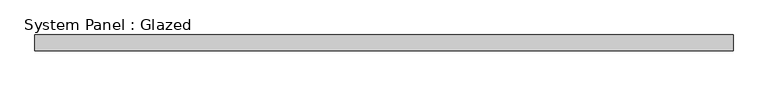
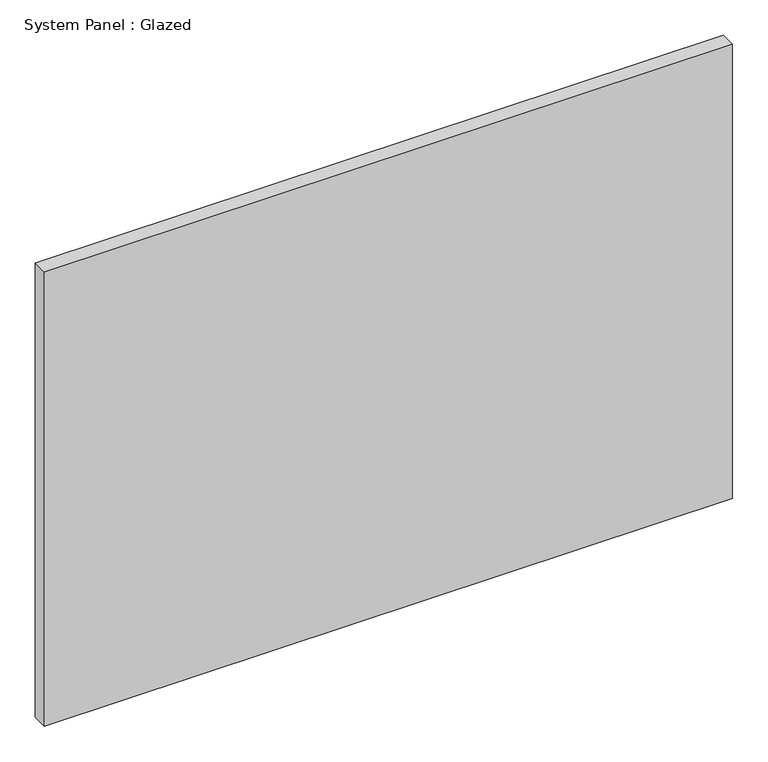
"""IFC4 building model written with IfcOpenShell, lengths in millimetres: plate geometry, System Panel : Glazed."""

from ifc_helpers import new_model, si_unit, origin, origin_with_axes, place, context, project, spatial, polyline, outline, extrude, source, transform, mapped, element, save


def system_panel_glazed_98635403(model_context):
    return source(origin(), model_context, "Body", "SweptSolid", [
        extrude(outline(polyline([(561.975, 19.05), (-561.975, 19.05), (-561.975, 44.45), (561.975, 44.45), (561.975, 19.05)])), origin_with_axes(), (0.0, 0.0, 1.0), 784.5104839),
    ])


if __name__ == "__main__":
    model = new_model("IFC4")
    model_context = context("Model", 3, world=origin())
    ifc_project = project(units=[si_unit("LENGTHUNIT", "METRE", prefix="MILLI")], contexts=[model_context])
    site = spatial("IfcSite", under=ifc_project)
    building = spatial("IfcBuilding", under=site)
    placement = place(None, origin())
    system_panel_glazed_shape = system_panel_glazed_98635403(model_context)
    element("IfcPlate", 1, ObjectType="System Panel : Glazed", at=placement, inside=building, context=model_context, shape_type="MappedRepresentation", body=[
        mapped(system_panel_glazed_shape, transform((0.0, 0.0, 0.0), x_axis=(1.0, 0.0, 0.0), y_axis=(0.0, 1.0, 0.0), z_axis=(0.0, 0.0, 1.0))),
    ])
    save(model, "model.ifc")

# Revit data of these elements
# Type "System Panel : Glazed"
#   Construction Type Id = "GSP4R"
#   Analytic Construction = "1/8 in Pilkington single glazing"
#   Visual Light Transmittance = 0.9
#   Solar Heat Gain Coefficient = 0.86
#   Heat Transfer Coefficient (U) = 1.18115 BTU/(h·ft²·°F)
#   Define Thermal Properties by = 1
# Element 1 (IfcPlate, "System Panel : Glazed")
#   Materials on its faces: "Glass"
# Materials
#   "Glass": class "Glass", colour RGB 0 128 192, transparency 0.75, Description = "Soda Lime Glass", Cost = 0
